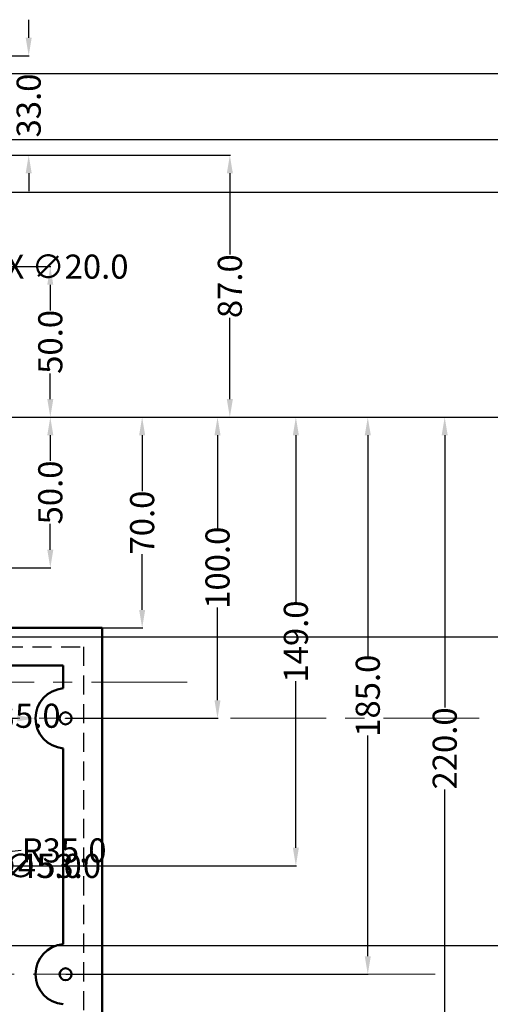
# Model space of a CAD drawing. Units: inches. Extents: x 11765 to 12471, y 10149 to 10793.
# Tile 7 of 8: x 12076 to 12232, y 10397 to 10724. Entities that reach past the tile are written whole.
import ezdxf

# ---------------------------------------------------------------- set-up
doc = ezdxf.new("R2010")
doc.units = ezdxf.units.IN
doc.header["$MEASUREMENT"] = 0
doc.linetypes.add('CENTER', pattern=[50.8, 31.75, -6.35, 6.35, -6.35])
doc.linetypes.add('HIDDEN', pattern=[9.525, 6.35, -3.175])
for name, color, linetype, lineweight in [('M-CNTR', 30, 'CENTER', 18), ('M-DIMS', 2, 'Continuous', 25), ('M-HIDN', 41, 'HIDDEN', 25), ('M-OUTL', 7, 'Continuous', 50)]:
    doc.layers.add(name, color=color, linetype=linetype, lineweight=lineweight)
doc.styles.get("Standard").update_dxf_attribs({"font": 'arial.ttf'})
doc.dimstyles.get("Standard").update_dxf_attribs({"dimtxt": 8, "dimasz": 6, "dimexe": 0.18, "dimexo": 0.0625, "dimgap": 0.09, "dimtad": 0, "dimtoh": 1, "dimdec": 1, "dimzin": 0, "dimdsep": 46, "dimtxsty": 'Standard', "dimcen": 0.09, "dimadec": 0, "dimazin": 0, "dimtfac": 1, "dimtdec": 1, "dimtofl": 0, "dimtmove": 0, "dimatfit": 3, "dimfxl": 1, "dimtolj": 1, "dimtzin": 0, "dimarcsym": 0})

# ---------------------------------------------------------------- blocks, each defined once
blk = doc.blocks.new('*D7')
at = {"layer": 'Defpoints', "color": 0, "transparency": 16777216}
for p in [(12066.91, 10679.15), (12145.22, 10679.15), (12066.91, 10592.15)]:
    blk.add_point(p, dxfattribs=at)
at = {"layer": 'M-DIMS', "color": 0, "lineweight": -2, "transparency": 16777216}
for p, q in [((12066.97, 10679.15), (12145.4, 10679.15)), ((12145.22, 10673.15), (12145.22, 10646.12)), ((12145.22, 10598.15), (12145.22, 10625.17)), ((12066.97, 10592.15), (12145.4, 10592.15))]:
    blk.add_line(p, q, dxfattribs=at)
at = {"layer": 'M-DIMS', "color": 0, "transparency": 16777216}
for points in [[(12144.22, 10673.15), (12146.22, 10673.15), (12145.22, 10679.15)], [(12144.22, 10598.15), (12146.22, 10598.15), (12145.22, 10592.15)]]:
    blk.add_solid(points, dxfattribs=at)
at = {"layer": 'M-DIMS', "color": 0, "transparency": 16777216, "insert": (12145.22, 10635.65), "char_height": 8, "attachment_point": 5, "rotation": 90}
blk.add_mtext('\\A1;87.0', dxfattribs=at)
blk = doc.blocks.new('*D8')
at = {"layer": 'Defpoints', "color": 0, "transparency": 16777216}
for p in [(12042.91, 10642.15), (12042.91, 10592.15), (12085.66, 10592.15)]:
    blk.add_point(p, dxfattribs=at)
at = {"layer": 'M-DIMS', "color": 0, "lineweight": -2, "transparency": 16777216}
for p, q in [((12042.97, 10642.15), (12085.84, 10642.15)), ((12085.66, 10636.15), (12085.66, 10627.61)), ((12085.66, 10598.15), (12085.66, 10606.68)), ((12042.97, 10592.15), (12085.84, 10592.15))]:
    blk.add_line(p, q, dxfattribs=at)
at = {"layer": 'M-DIMS', "color": 0, "transparency": 16777216}
for points in [[(12084.66, 10636.15), (12086.66, 10636.15), (12085.66, 10642.15)], [(12084.66, 10598.15), (12086.66, 10598.15), (12085.66, 10592.15)]]:
    blk.add_solid(points, dxfattribs=at)
at = {"layer": 'M-DIMS', "color": 0, "transparency": 16777216, "insert": (12085.66, 10617.15), "char_height": 8, "attachment_point": 5, "rotation": 90}
blk.add_mtext('\\A1;50.0', dxfattribs=at)
blk = doc.blocks.new('*D9')
at = {"layer": 'Defpoints', "color": 0, "transparency": 16777216}
for p in [(12042.91, 10592.15), (12085.66, 10592.15), (12042.91, 10542.15)]:
    blk.add_point(p, dxfattribs=at)
at = {"layer": 'M-DIMS', "color": 0, "lineweight": -2, "transparency": 16777216}
for p, q in [((12042.97, 10592.15), (12085.84, 10592.15)), ((12085.66, 10586.15), (12085.66, 10577.61)), ((12085.66, 10548.15), (12085.66, 10556.68)), ((12042.97, 10542.15), (12085.84, 10542.15))]:
    blk.add_line(p, q, dxfattribs=at)
at = {"layer": 'M-DIMS', "color": 0, "transparency": 16777216}
for points in [[(12084.66, 10586.15), (12086.66, 10586.15), (12085.66, 10592.15)], [(12084.66, 10548.15), (12086.66, 10548.15), (12085.66, 10542.15)]]:
    blk.add_solid(points, dxfattribs=at)
at = {"layer": 'M-DIMS', "color": 0, "transparency": 16777216, "insert": (12085.66, 10567.15), "char_height": 8, "attachment_point": 5, "rotation": 90}
blk.add_mtext('\\A1;50.0', dxfattribs=at)
blk = doc.blocks.new('*D10')
at = {"layer": 'Defpoints', "color": 0, "transparency": 16777216}
for p in [(12102.91, 10592.15), (12116.13, 10592.15), (12102.91, 10522.15)]:
    blk.add_point(p, dxfattribs=at)
at = {"layer": 'M-DIMS', "color": 0, "lineweight": -2, "transparency": 16777216}
for p, q in [((12102.97, 10592.15), (12116.31, 10592.15)), ((12116.13, 10586.15), (12116.13, 10567.58)), ((12116.13, 10528.15), (12116.13, 10546.71)), ((12102.97, 10522.15), (12116.31, 10522.15))]:
    blk.add_line(p, q, dxfattribs=at)
at = {"layer": 'M-DIMS', "color": 0, "transparency": 16777216}
for points in [[(12115.13, 10586.15), (12117.13, 10586.15), (12116.13, 10592.15)], [(12115.13, 10528.15), (12117.13, 10528.15), (12116.13, 10522.15)]]:
    blk.add_solid(points, dxfattribs=at)
at = {"layer": 'M-DIMS', "color": 0, "transparency": 16777216, "insert": (12116.13, 10557.15), "char_height": 8, "attachment_point": 5, "rotation": 90}
blk.add_mtext('\\A1;70.0', dxfattribs=at)
blk = doc.blocks.new('*D11')
at = {"layer": 'Defpoints', "color": 0, "transparency": 16777216}
for p in [(12090.75, 10592.15), (12141.13, 10592.15), (12090.75, 10492.15)]:
    blk.add_point(p, dxfattribs=at)
at = {"layer": 'M-DIMS', "color": 0, "lineweight": -2, "transparency": 16777216}
for p, q in [((12090.81, 10592.15), (12141.31, 10592.15)), ((12141.13, 10586.15), (12141.13, 10555.34)), ((12141.13, 10498.15), (12141.13, 10528.95)), ((12090.81, 10492.15), (12141.31, 10492.15))]:
    blk.add_line(p, q, dxfattribs=at)
at = {"layer": 'M-DIMS', "color": 0, "transparency": 16777216}
for points in [[(12140.13, 10586.15), (12142.13, 10586.15), (12141.13, 10592.15)], [(12140.13, 10498.15), (12142.13, 10498.15), (12141.13, 10492.15)]]:
    blk.add_solid(points, dxfattribs=at)
at = {"layer": 'M-DIMS', "color": 0, "transparency": 16777216, "insert": (12141.13, 10542.15), "char_height": 8, "attachment_point": 5, "rotation": 90}
blk.add_mtext('\\A1;100.0', dxfattribs=at)
blk = doc.blocks.new('*D12')
at = {"layer": 'Defpoints', "color": 0, "transparency": 16777216}
for p in [(12130.14, 10592.15), (12029.23, 10443.15), (12167.12, 10443.15)]:
    blk.add_point(p, dxfattribs=at)
at = {"layer": 'M-DIMS', "color": 0, "lineweight": -2, "transparency": 16777216}
for p, q in [((12130.2, 10592.15), (12167.3, 10592.15)), ((12167.12, 10586.15), (12167.12, 10530.84)), ((12167.12, 10449.15), (12167.12, 10504.45)), ((12029.29, 10443.15), (12167.3, 10443.15))]:
    blk.add_line(p, q, dxfattribs=at)
at = {"layer": 'M-DIMS', "color": 0, "transparency": 16777216}
for points in [[(12166.12, 10586.15), (12168.12, 10586.15), (12167.12, 10592.15)], [(12166.12, 10449.15), (12168.12, 10449.15), (12167.12, 10443.15)]]:
    blk.add_solid(points, dxfattribs=at)
at = {"layer": 'M-DIMS', "color": 0, "transparency": 16777216, "insert": (12167.12, 10517.65), "char_height": 8, "attachment_point": 5, "rotation": 90}
blk.add_mtext('\\A1;149.0', dxfattribs=at)
blk = doc.blocks.new('*D13')
at = {"layer": 'Defpoints', "color": 0, "transparency": 16777216}
for p in [(12156.23, 10592.15), (12090.75, 10407.15), (12190.98, 10407.15)]:
    blk.add_point(p, dxfattribs=at)
at = {"layer": 'M-DIMS', "color": 0, "lineweight": -2, "transparency": 16777216}
for p, q in [((12156.3, 10592.15), (12191.16, 10592.15)), ((12190.98, 10586.15), (12190.98, 10512.84)), ((12190.98, 10413.15), (12190.98, 10486.45)), ((12090.81, 10407.15), (12191.16, 10407.15))]:
    blk.add_line(p, q, dxfattribs=at)
at = {"layer": 'M-DIMS', "color": 0, "transparency": 16777216}
for points in [[(12189.98, 10586.15), (12191.98, 10586.15), (12190.98, 10592.15)], [(12189.98, 10413.15), (12191.98, 10413.15), (12190.98, 10407.15)]]:
    blk.add_solid(points, dxfattribs=at)
at = {"layer": 'M-DIMS', "color": 0, "transparency": 16777216, "insert": (12190.98, 10499.65), "char_height": 8, "attachment_point": 5, "rotation": 90}
blk.add_mtext('\\A1;185.0', dxfattribs=at)
blk = doc.blocks.new('*D14')
at = {"layer": 'Defpoints', "color": 0, "transparency": 16777216}
for p in [(12156.23, 10592.15), (12216.5, 10592.15), (11992.91, 10372.15)]:
    blk.add_point(p, dxfattribs=at)
at = {"layer": 'M-DIMS', "color": 0, "lineweight": -2, "transparency": 16777216}
for p, q in [((12156.3, 10592.15), (12216.68, 10592.15)), ((12216.5, 10586.15), (12216.5, 10495.79)), ((12216.5, 10378.15), (12216.5, 10468.5)), ((11992.97, 10372.15), (12216.68, 10372.15))]:
    blk.add_line(p, q, dxfattribs=at)
at = {"layer": 'M-DIMS', "color": 0, "transparency": 16777216}
for points in [[(12215.5, 10586.15), (12217.5, 10586.15), (12216.5, 10592.15)], [(12215.5, 10378.15), (12217.5, 10378.15), (12216.5, 10372.15)]]:
    blk.add_solid(points, dxfattribs=at)
at = {"layer": 'M-DIMS', "color": 0, "transparency": 16777216, "insert": (12216.5, 10482.15), "char_height": 8, "attachment_point": 5, "rotation": 90}
blk.add_mtext('\\A1;220.0', dxfattribs=at)
blk = doc.blocks.new('*D15')
at = {"layer": 'Defpoints', "color": 0, "transparency": 16777216}
for p in [(12198.7, 10592.15), (12090.75, 10322.15), (12241.87, 10322.15)]:
    blk.add_point(p, dxfattribs=at)
at = {"layer": 'M-DIMS', "color": 0, "lineweight": -2, "transparency": 16777216}
for p, q in [((12198.76, 10592.15), (12242.05, 10592.15)), ((12241.87, 10586.15), (12241.87, 10470.79)), ((12241.87, 10328.15), (12241.87, 10443.5)), ((12090.81, 10322.15), (12242.05, 10322.15))]:
    blk.add_line(p, q, dxfattribs=at)
at = {"layer": 'M-DIMS', "color": 0, "transparency": 16777216}
for points in [[(12240.87, 10586.15), (12242.87, 10586.15), (12241.87, 10592.15)], [(12240.87, 10328.15), (12242.87, 10328.15), (12241.87, 10322.15)]]:
    blk.add_solid(points, dxfattribs=at)
at = {"layer": 'M-DIMS', "color": 0, "transparency": 16777216, "insert": (12241.87, 10457.15), "char_height": 8, "attachment_point": 5, "rotation": 90}
blk.add_mtext('\\A1;270.0', dxfattribs=at)
blk = doc.blocks.new('*D28')
at = {"layer": 'Defpoints', "color": 0, "transparency": 16777216}
for p in [(12053.91, 10712.15), (12078.49, 10712.15), (12053.91, 10679.15)]:
    blk.add_point(p, dxfattribs=at)
at = {"layer": 'M-DIMS', "color": 0, "lineweight": -2, "transparency": 16777216}
for p, q in [((12078.49, 10718.15), (12078.49, 10724.15)), ((12053.97, 10712.15), (12078.67, 10712.15)), ((12053.97, 10679.15), (12078.67, 10679.15)), ((12078.49, 10673.15), (12078.49, 10667.15))]:
    blk.add_line(p, q, dxfattribs=at)
at = {"layer": 'M-DIMS', "color": 0, "transparency": 16777216}
for points in [[(12077.49, 10718.15), (12079.49, 10718.15), (12078.49, 10712.15)], [(12077.49, 10673.15), (12079.49, 10673.15), (12078.49, 10679.15)]]:
    blk.add_solid(points, dxfattribs=at)
at = {"layer": 'M-DIMS', "color": 0, "transparency": 16777216, "insert": (12078.49, 10695.65), "char_height": 8, "attachment_point": 5, "rotation": 90}
blk.add_mtext('\\A1;33.0', dxfattribs=at)
blk = doc.blocks.new('*D46')
at = {"layer": 'Defpoints', "color": 0, "transparency": 16777216}
for p in [(12064.02, 10446.97), (12029.23, 10443.15)]:
    blk.add_point(p, dxfattribs=at)
at = {"layer": 'M-DIMS', "color": 0, "lineweight": -2, "transparency": 16777216}
for p, q in [((12075.95, 10448.28), (12069.99, 10447.62)), ((12029.14, 10443.15), (12029.32, 10443.15)), ((12029.23, 10443.06), (12029.23, 10443.24))]:
    blk.add_line(p, q, dxfattribs=at)
at = {"layer": 'M-DIMS', "color": 0, "transparency": 16777216}
blk.add_solid([(12069.88, 10448.62), (12070.1, 10446.63), (12064.02, 10446.97)], dxfattribs=at)
at = {"layer": 'M-DIMS', "color": 0, "transparency": 16777216, "insert": (12090.25, 10448.28), "char_height": 8, "attachment_point": 5}
blk.add_mtext('\\A1;R35.0', dxfattribs=at)
blk = doc.blocks.new('*D62')
at = {"layer": 'Defpoints', "color": 0, "transparency": 16777216}
for p in [(12379.9, 10706.15), (11848.16, 10684.29), (12385.4, 10684.29)]:
    blk.add_point(p, dxfattribs=at)
at = {"layer": 'M-DIMS', "color": 0, "lineweight": -2, "transparency": 16777216}
for p, q in [((12379.83, 10706.15), (11847.98, 10706.15)), ((11848.16, 10700.15), (11848.16, 10690.29)), ((12385.33, 10684.29), (11847.98, 10684.29)), ((11848.16, 10684.29), (11848.16, 10678.29)), ((11848.16, 10678.29), (11842.16, 10678.29))]:
    blk.add_line(p, q, dxfattribs=at)
at = {"layer": 'M-DIMS', "color": 0, "transparency": 16777216}
for points in [[(11847.16, 10700.15), (11849.16, 10700.15), (11848.16, 10706.15)], [(11847.16, 10690.29), (11849.16, 10690.29), (11848.16, 10684.29)]]:
    blk.add_solid(points, dxfattribs=at)
at = {"layer": 'M-DIMS', "color": 0, "transparency": 16777216, "insert": (11828.51, 10678.29), "char_height": 8, "attachment_point": 5}
blk.add_mtext('\\A1;21.86', dxfattribs=at)
blk = doc.blocks.new('*D63')
at = {"layer": 'Defpoints', "color": 0, "transparency": 16777216}
for p in [(12385.4, 10684.29), (11848.16, 10666.79), (12385.4, 10666.79)]:
    blk.add_point(p, dxfattribs=at)
at = {"layer": 'M-DIMS', "color": 0, "lineweight": -2, "transparency": 16777216}
for p, q in [((12385.33, 10684.29), (11847.98, 10684.29)), ((11848.16, 10678.29), (11848.16, 10672.79)), ((12385.33, 10666.79), (11847.98, 10666.79)), ((11848.16, 10666.79), (11848.16, 10660.79)), ((11848.16, 10660.79), (11842.16, 10660.79))]:
    blk.add_line(p, q, dxfattribs=at)
at = {"layer": 'M-DIMS', "color": 0, "transparency": 16777216}
for points in [[(11847.16, 10678.29), (11849.16, 10678.29), (11848.16, 10684.29)], [(11847.16, 10672.79), (11849.16, 10672.79), (11848.16, 10666.79)]]:
    blk.add_solid(points, dxfattribs=at)
at = {"layer": 'M-DIMS', "color": 0, "transparency": 16777216, "insert": (11832.03, 10660.79), "char_height": 8, "attachment_point": 5}
blk.add_mtext('\\A1;17.5', dxfattribs=at)
blk = doc.blocks.new('*D66')
at = {"layer": 'Defpoints', "color": 0, "transparency": 16777216}
for p in [(12386.9, 10519.15), (11848.16, 10416.65), (12386.9, 10416.65)]:
    blk.add_point(p, dxfattribs=at)
at = {"layer": 'M-DIMS', "color": 0, "lineweight": -2, "transparency": 16777216}
for p, q in [((12386.83, 10519.15), (11847.98, 10519.15)), ((11848.16, 10513.15), (11848.16, 10481.14)), ((11848.16, 10422.65), (11848.16, 10454.65)), ((12386.83, 10416.65), (11847.98, 10416.65))]:
    blk.add_line(p, q, dxfattribs=at)
at = {"layer": 'M-DIMS', "color": 0, "transparency": 16777216}
for points in [[(11847.16, 10513.15), (11849.16, 10513.15), (11848.16, 10519.15)], [(11847.16, 10422.65), (11849.16, 10422.65), (11848.16, 10416.65)]]:
    blk.add_solid(points, dxfattribs=at)
at = {"layer": 'M-DIMS', "color": 0, "transparency": 16777216, "insert": (11848.16, 10467.9), "char_height": 8, "attachment_point": 5, "rotation": 90}
blk.add_mtext('\\A1;102.5', dxfattribs=at)
blk = doc.blocks.new('*D71')
at = {"layer": 'Defpoints', "color": 0, "transparency": 16777216}
for p in [(12045.17, 10474.31), (12029.23, 10443.15)]:
    blk.add_point(p, dxfattribs=at)
at = {"layer": 'M-DIMS', "color": 0, "lineweight": -2, "transparency": 16777216}
for p, q in [((12054.74, 10493), (12047.9, 10479.65)), ((12060.74, 10493), (12054.74, 10493)), ((12029.14, 10443.15), (12029.32, 10443.15)), ((12029.23, 10443.06), (12029.23, 10443.24))]:
    blk.add_line(p, q, dxfattribs=at)
at = {"layer": 'M-DIMS', "color": 0, "transparency": 16777216}
blk.add_solid([(12047.01, 10480.1), (12048.79, 10479.19), (12045.17, 10474.31)], dxfattribs=at)
at = {"layer": 'M-DIMS', "color": 0, "transparency": 16777216, "insert": (12075.03, 10493), "char_height": 8, "attachment_point": 5}
blk.add_mtext('\\A1;R35.0', dxfattribs=at)
blk = doc.blocks.new('*D73')
at = {"layer": 'Defpoints', "color": 0, "transparency": 16777216}
for p in [(12002.73, 10443.15), (12055.73, 10443.15)]:
    blk.add_point(p, dxfattribs=at)
at = {"layer": 'M-DIMS', "color": 0, "lineweight": -2, "transparency": 16777216}
for p, q in [((12029.14, 10443.15), (12029.32, 10443.15)), ((12029.23, 10443.06), (12029.23, 10443.24)), ((12071.63, 10443.15), (12061.73, 10443.15))]:
    blk.add_line(p, q, dxfattribs=at)
at = {"layer": 'M-DIMS', "color": 0, "transparency": 16777216}
blk.add_solid([(12061.73, 10444.15), (12061.73, 10442.15), (12055.73, 10443.15)], dxfattribs=at)
at = {"layer": 'M-DIMS', "color": 0, "transparency": 16777216, "insert": (12086.45, 10443.15), "char_height": 8, "attachment_point": 5}
blk.add_mtext('\\A1;∅53.0', dxfattribs=at)
blk = doc.blocks.new('*D74')
at = {"layer": 'Defpoints', "color": 0, "transparency": 16777216}
for p in [(12006.73, 10443.15), (12051.73, 10443.15)]:
    blk.add_point(p, dxfattribs=at)
at = {"layer": 'M-DIMS', "color": 0, "lineweight": -2, "transparency": 16777216}
for p, q in [((12029.14, 10443.15), (12029.32, 10443.15)), ((12029.23, 10443.06), (12029.23, 10443.24)), ((12065.23, 10443.15), (12057.73, 10443.15))]:
    blk.add_line(p, q, dxfattribs=at)
at = {"layer": 'M-DIMS', "color": 0, "transparency": 16777216}
blk.add_solid([(12057.73, 10444.15), (12057.73, 10442.15), (12051.73, 10443.15)], dxfattribs=at)
at = {"layer": 'M-DIMS', "color": 0, "transparency": 16777216, "insert": (12080.05, 10443.15), "char_height": 8, "attachment_point": 5}
blk.add_mtext('\\A1;∅45.0', dxfattribs=at)
blk = doc.blocks.new('*D79')
at = {"layer": 'Defpoints', "color": 0, "transparency": 16777216}
for p in [(12080.75, 10492.15), (12090.75, 10492.15)]:
    blk.add_point(p, dxfattribs=at)
at = {"layer": 'M-DIMS', "color": 0, "lineweight": -2, "transparency": 16777216}
for p, q in [((12068.75, 10492.15), (12074.75, 10492.15)), ((12090.66, 10492.15), (12090.84, 10492.15)), ((12090.75, 10492.06), (12090.75, 10492.24))]:
    blk.add_line(p, q, dxfattribs=at)
at = {"layer": 'M-DIMS', "color": 0, "transparency": 16777216}
blk.add_solid([(12074.75, 10493.15), (12074.75, 10491.15), (12080.75, 10492.15)], dxfattribs=at)
at = {"layer": 'M-DIMS', "color": 0, "transparency": 16777216, "insert": (12045.85, 10492.15), "char_height": 8, "attachment_point": 5}
blk.add_mtext('\\A1;8X R10.0', dxfattribs=at)
blk = doc.blocks.new('*D80')
at = {"layer": 'Defpoints', "color": 0, "transparency": 16777216}
for p in [(12032.91, 10642.15), (12052.91, 10642.15)]:
    blk.add_point(p, dxfattribs=at)
at = {"layer": 'M-DIMS', "color": 0, "lineweight": -2, "transparency": 16777216}
for p, q in [((12042.82, 10642.15), (12043, 10642.15)), ((12042.91, 10642.06), (12042.91, 10642.24)), ((12064.91, 10642.15), (12058.91, 10642.15))]:
    blk.add_line(p, q, dxfattribs=at)
at = {"layer": 'M-DIMS', "color": 0, "transparency": 16777216}
blk.add_solid([(12058.91, 10643.15), (12058.91, 10641.15), (12052.91, 10642.15)], dxfattribs=at)
at = {"layer": 'M-DIMS', "color": 0, "transparency": 16777216, "insert": (12088.18, 10642.15), "char_height": 8, "attachment_point": 5}
blk.add_mtext('\\A1;2X ∅20.0', dxfattribs=at)

msp = doc.modelspace()

# ---------------------------------------------------------------- linework, layer by layer
at = {"layer": 'M-CNTR'}
for p, q in [((12131.07, 10504.146), (11882.912, 10504.146)), ((12227.966, 10492.146), (11882.912, 10492.146)), ((12213.332, 10407.146), (11882.912, 10407.146))]:
    msp.add_line(p, q, dxfattribs=at)
at = {"layer": 'M-HIDN'}
msp.add_lwpolyline([(12060.662, 10705.896), (12060.662, 10515.896), (12096.662, 10515.896), (12096.662, 10263.352), (12062.096, 10243.396), (11923.728, 10243.396), (11889.162, 10263.352), (11889.162, 10705.896)], close=True, dxfattribs=at)
at = {"layer": 'M-OUTL'}
for p, q in [((12102.912, 10522.146), (12066.912, 10522.146)), ((12102.912, 10257.146), (12102.912, 10522.146)), ((12089.912, 10509.646), (12053.912, 10509.646)), ((12089.912, 10502.111), (12089.912, 10509.646)), ((12089.912, 10417.111), (12089.912, 10482.181))]:
    msp.add_line(p, q, dxfattribs=at)
for centre in [(12090.748, 10492.146), (12090.748, 10407.146)]:
    msp.add_circle(centre, 2, dxfattribs=at)
for centre in [(12090.748, 10492.146), (12090.748, 10407.146)]:
    msp.add_arc(centre, 10, 94.79487, 265.20513, dxfattribs=at)

# ---------------------------------------------------------------- dimensions: what is measured, and where the dimension line sits
at = {"layer": 'M-DIMS'}
for base, p1, p2, override, picture, middle in [((12078.487, 10712.146), (12053.912, 10679.146), (12053.912, 10712.146), {"dimclrd": 0, "dimclre": 0, "dimclrt": 0}, '*D28', (12078.487, 10695.646)), ((11848.162, 10684.286), (12379.896, 10706.146), (12385.396, 10684.286), {"dimdec": 2, "dimlfac": 1, "dimrnd": 0, "dimzin": 0, "dimdsep": 46, "dimlunit": 2}, '*D62', (11828.509, 10678.286)), ((11848.162, 10666.786), (12385.396, 10684.286), (12385.396, 10666.786), {"dimdec": 1, "dimlfac": 1, "dimrnd": 0, "dimzin": 0, "dimdsep": 46, "dimlunit": 2}, '*D63', (11832.028, 10660.786)), ((12145.224, 10679.146), (12066.912, 10592.146), (12066.912, 10679.146), {"dimclrd": 0, "dimclre": 0, "dimclrt": 0}, '*D7', (12145.224, 10635.646)), ((12085.657, 10592.146), (12042.912, 10642.146), (12042.912, 10592.146), {"dimclrd": 0, "dimclre": 0, "dimclrt": 0}, '*D8', (12085.657, 10617.146)), ((12216.505, 10592.146), (11992.912, 10372.146), (12156.234, 10592.146), {"dimclrd": 0, "dimclre": 0, "dimclrt": 0}, '*D14', (12216.505, 10482.146)), ((12167.122, 10443.146), (12130.138, 10592.146), (12029.232, 10443.146), {"dimclrd": 0, "dimclre": 0, "dimclrt": 0}, '*D12', (12167.122, 10517.646)), ((12085.657, 10592.146), (12042.912, 10542.146), (12042.912, 10592.146), {"dimclrd": 0, "dimclre": 0, "dimclrt": 0}, '*D9', (12085.657, 10567.146)), ((12141.133, 10592.146), (12090.748, 10492.146), (12090.748, 10592.146), {"dimclrd": 0, "dimclre": 0, "dimclrt": 0}, '*D11', (12141.133, 10542.146)), ((12190.98, 10407.146), (12156.234, 10592.146), (12090.748, 10407.146), {"dimclrd": 0, "dimclre": 0, "dimclrt": 0}, '*D13', (12190.98, 10499.646)), ((12241.874, 10322.146), (12198.696, 10592.146), (12090.748, 10322.146), {"dimclrd": 0, "dimclre": 0, "dimclrt": 0}, '*D15', (12241.874, 10457.146)), ((12116.129, 10592.146), (12102.912, 10522.146), (12102.912, 10592.146), {"dimclrd": 0, "dimclre": 0, "dimclrt": 0}, '*D10', (12116.129, 10557.146)), ((11848.162, 10416.646), (12386.896, 10519.146), (12386.896, 10416.646), {"dimdec": 1, "dimlfac": 1, "dimrnd": 0, "dimzin": 0, "dimdsep": 46, "dimlunit": 2}, '*D66', (11848.162, 10467.896))]:
    dim = msp.add_linear_dim(base=base, p1=p1, p2=p2, angle=90, dimstyle='Standard', override=override, dxfattribs=at)
    dim.commit()
    dim.dimension.update_dxf_attribs({"geometry": picture, "text_midpoint": middle})
dim = msp.add_diameter_dim_2p(p1=(12032.912, 10642.145), p2=(12052.912, 10642.146), text='2X <>', dimstyle='Standard', override={"dimdec": 1, "dimlfac": 1, "dimrnd": 0, "dimzin": 0, "dimdsep": 46, "dimlunit": 2}, dxfattribs=at)
dim.commit()
dim.dimension.update_dxf_attribs({"geometry": '*D80', "text_midpoint": (12064.912, 10642.147)})
dim = msp.add_radius_dim(center=(12090.748, 10492.146), mpoint=(12080.748, 10492.15), text='8X <>', dimstyle='Standard', override={"dimdec": 1, "dimlfac": 1, "dimrnd": 0, "dimzin": 0, "dimdsep": 46, "dimlunit": 2}, dxfattribs=at)
dim.commit()
dim.dimension.update_dxf_attribs({"geometry": '*D79', "text_midpoint": (12045.853, 10492.155)})
dim = msp.add_radius_dim(center=(12029.232, 10443.146), mpoint=(12045.172, 10474.305), dimstyle='Standard', override={"dimdec": 1, "dimlfac": 1, "dimrnd": 0, "dimzin": 0, "dimdsep": 46, "dimlunit": 2}, dxfattribs=at)
dim.commit()
dim.dimension.update_dxf_attribs({"geometry": '*D71', "text_midpoint": (12075.031, 10493.001), "dimtype": 164})
dim = msp.add_radius_dim(center=(12029.232, 10443.146), mpoint=(12064.023, 10446.969), dimstyle='Standard', override={"dimclrd": 0, "dimclre": 0, "dimclrt": 0}, dxfattribs=at)
dim.commit()
dim.dimension.update_dxf_attribs({"geometry": '*D46', "text_midpoint": (12090.245, 10448.28)})
for p1, p2, picture, middle in [((12002.732, 10443.145), (12055.732, 10443.146), '*D73', (12071.632, 10443.146)), ((12006.732, 10443.145), (12051.732, 10443.146), '*D74', (12065.232, 10443.146))]:
    dim = msp.add_diameter_dim_2p(p1=p1, p2=p2, dimstyle='Standard', override={"dimdec": 1, "dimlfac": 1, "dimrnd": 0, "dimzin": 0, "dimdsep": 46, "dimlunit": 2}, dxfattribs=at)
    dim.commit()
    dim.dimension.update_dxf_attribs({"geometry": picture, "text_midpoint": middle, "dimtype": 163})

doc.saveas('drawing.dxf')
